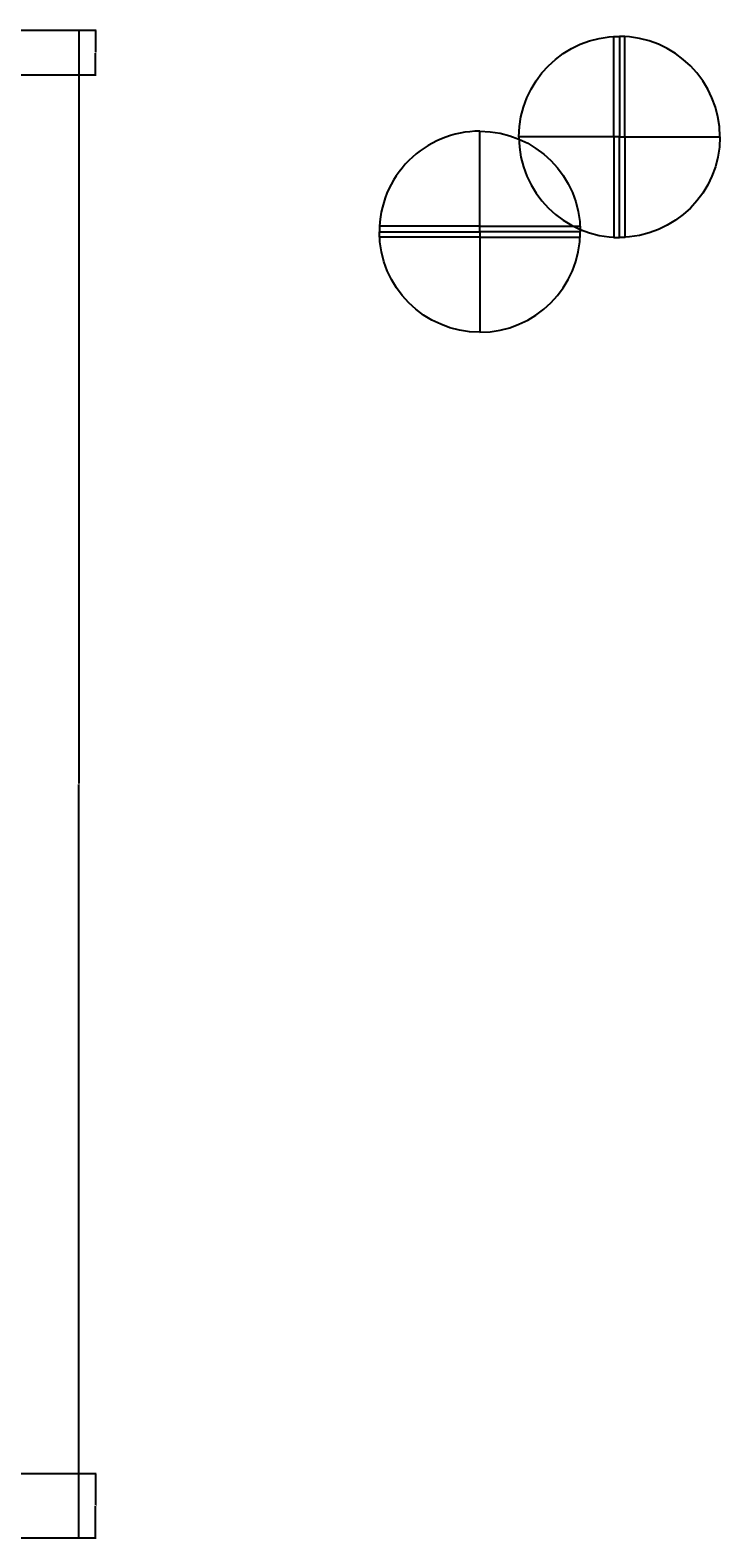
# Model space of a CAD drawing. Units: inches. Extents: x 224 to 929, y 339 to 940.
# Tile 3 of 3: x 682 to 929, y 370 to 910. Entities that reach past the tile are written whole.
import ezdxf

# ---------------------------------------------------------------- set-up
doc = ezdxf.new("R2010")
doc.units = ezdxf.units.IN
doc.layers.add('A-ANNO-DIMS', color=2, linetype='Continuous', lineweight=18)
doc.layers.add('A-DOOR', color=3, linetype='Continuous', lineweight=25)
doc.styles.get("Standard").update_dxf_attribs({"font": 'arial.ttf'})
doc.dimstyles.get("Standard").update_dxf_attribs({"dimtxt": 0.18, "dimasz": 0.18, "dimexe": 0.18, "dimexo": 0.0625, "dimgap": 0.09, "dimtad": 0, "dimtih": 1, "dimtoh": 1, "dimdec": 4, "dimzin": 0, "dimdsep": 46, "dimtxsty": 'Standard', "dimcen": 0.09, "dimadec": 0, "dimazin": 0, "dimtfac": 1, "dimtdec": 4, "dimtofl": 0, "dimtmove": 0, "dimatfit": 3, "dimfxl": 1, "dimtolj": 1, "dimtzin": 0, "dimarcsym": 0})

# ---------------------------------------------------------------- blocks, each defined once
blk = doc.blocks.new('DOOR-SINGLE-36IN')
blk.add_line((0, 0), (36, 0))
blk.add_lwpolyline([(2, 0), (2, 36), (0, 36), (0, 0)], close=True)
blk.add_arc((0, 0), 36, 0, 90)
blk = doc.blocks.new('*D16')
at = {"layer": 'A-ANNO-DIMS', "color": 0, "lineweight": -2, "transparency": 16777216}
for p, q in [((668.73, 909.63), (699.35, 909.63)), ((699.17, 909.45), (699.17, 639.81)), ((699.17, 369.81), (699.17, 639.44)), ((668.73, 369.63), (699.35, 369.63))]:
    blk.add_line(p, q, dxfattribs=at)
at = {"layer": 'A-ANNO-DIMS', "color": 0, "transparency": 16777216}
for points in [[(699.14, 909.45), (699.2, 909.45), (699.17, 909.63)], [(699.14, 369.81), (699.2, 369.81), (699.17, 369.63)]]:
    blk.add_solid(points, dxfattribs=at)
at = {"layer": 'Defpoints', "color": 0, "transparency": 16777216}
for p in [(668.67, 909.63), (668.67, 369.63), (699.17, 369.63)]:
    blk.add_point(p, dxfattribs=at)
at = {"layer": 'A-ANNO-DIMS', "color": 0, "transparency": 16777216, "insert": (699.17, 639.63), "char_height": 0.18, "attachment_point": 5}
blk.add_mtext('\\A1;540', dxfattribs=at)
blk = doc.blocks.new('*D37')
at = {"layer": 'A-ANNO-DIMS', "color": 0, "lineweight": -2, "transparency": 16777216}
for p, q in [((668.73, 909.63), (705.35, 909.63)), ((705.17, 909.45), (705.17, 901.79)), ((705.17, 893.77), (705.17, 901.43)), ((649.94, 893.59), (705.35, 893.59))]:
    blk.add_line(p, q, dxfattribs=at)
at = {"layer": 'A-ANNO-DIMS', "color": 0, "transparency": 16777216}
for points in [[(705.14, 909.45), (705.2, 909.45), (705.17, 909.63)], [(705.14, 893.77), (705.2, 893.77), (705.17, 893.59)]]:
    blk.add_solid(points, dxfattribs=at)
at = {"layer": 'Defpoints', "color": 0, "transparency": 16777216}
for p in [(668.67, 909.63), (649.88, 893.59), (705.17, 893.59)]:
    blk.add_point(p, dxfattribs=at)
at = {"layer": 'A-ANNO-DIMS', "color": 0, "transparency": 16777216, "insert": (705.17, 901.61), "char_height": 0.18, "attachment_point": 5}
blk.add_mtext('\\A1;16.032', dxfattribs=at)
blk = doc.blocks.new('*D39')
at = {"layer": 'A-ANNO-DIMS', "color": 0, "lineweight": -2, "transparency": 16777216}
for p, q in [((660, 392.68), (705.35, 392.68)), ((705.17, 392.5), (705.17, 381.33)), ((705.17, 369.81), (705.17, 380.97)), ((668.73, 369.63), (705.35, 369.63))]:
    blk.add_line(p, q, dxfattribs=at)
at = {"layer": 'A-ANNO-DIMS', "color": 0, "transparency": 16777216}
for points in [[(705.14, 392.5), (705.2, 392.5), (705.17, 392.68)], [(705.14, 369.81), (705.2, 369.81), (705.17, 369.63)]]:
    blk.add_solid(points, dxfattribs=at)
at = {"layer": 'Defpoints', "color": 0, "transparency": 16777216}
for p in [(659.94, 392.68), (705.17, 392.68), (668.67, 369.63)]:
    blk.add_point(p, dxfattribs=at)
at = {"layer": 'A-ANNO-DIMS', "color": 0, "transparency": 16777216, "insert": (705.17, 381.15), "char_height": 0.18, "attachment_point": 5}
blk.add_mtext('\\A1;23.054', dxfattribs=at)

msp = doc.modelspace()

# ---------------------------------------------------------------- block references
at = {"layer": 'A-DOOR', "extrusion": (0, 0, -1), "zscale": -1}
msp.add_blockref('DOOR-SINGLE-36IN', (-892.8555, 871.3812), dxfattribs=at)
at = {"layer": 'A-DOOR'}
msp.add_blockref('DOOR-SINGLE-36IN', (892.8552, 871.3812), dxfattribs=at)
for p, rotation in [((842.8411, 837.4368), 89.99999999999962), ((892.8555, 871.3815), 180), ((842.8407, 837.4371), 270.0000000000001)]:
    msp.add_blockref('DOOR-SINGLE-36IN', p, dxfattribs=dict(at, rotation=rotation))
at = {"layer": 'A-DOOR', "extrusion": (0, 0, -1), "zscale": -1}
for p, rotation in [((-842.8407, 837.4368), 90.00000000000006), ((-892.8552, 871.3815), 180), ((-842.8411, 837.4371), 270.0000000000006)]:
    msp.add_blockref('DOOR-SINGLE-36IN', p, dxfattribs=dict(at, rotation=rotation))

# ---------------------------------------------------------------- dimensions: what is measured, and where the dimension line sits
at = {"layer": 'A-ANNO-DIMS'}
for base, p1, p2, angle, override, picture, middle in [((705.1661, 893.5934), (668.6661, 909.6252), (649.8759, 893.5934), 90, {"dimdec": 3, "dimlfac": 1, "dimrnd": 0, "dimzin": 0, "dimdsep": 46, "dimlunit": 2}, '*D37', (705.1661, 901.6093)), ((699.1661, 369.6252), (668.6661, 909.6252), (668.6661, 369.6252), 270, {"dimdec": 0, "dimlfac": 1, "dimrnd": 0, "dimzin": 0, "dimdsep": 46, "dimlunit": 2}, '*D16', (699.1661, 639.6252)), ((705.1661, 392.6791), (668.6661, 369.6252), (659.9364, 392.6791), 90, {"dimdec": 3, "dimlfac": 1, "dimrnd": 0, "dimzin": 0, "dimdsep": 46, "dimlunit": 2}, '*D39', (705.1661, 381.1521))]:
    dim = msp.add_linear_dim(base=base, p1=p1, p2=p2, angle=angle, dimstyle='Standard', override=override, dxfattribs=at)
    dim.commit()
    dim.dimension.update_dxf_attribs({"geometry": picture, "text_midpoint": middle})

doc.saveas('drawing.dxf')
